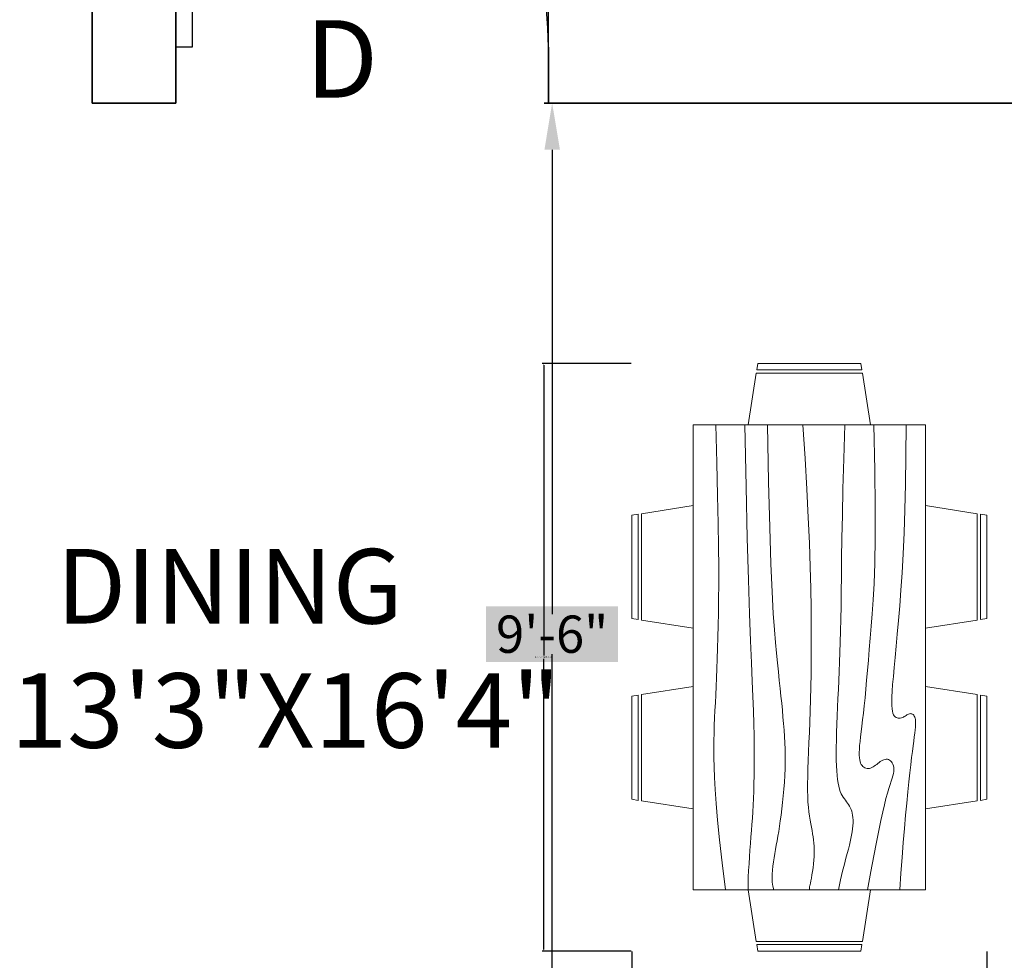
# Model space of a CAD drawing. Units: inches. Extents: x -128 to 854, y -395 to 398.
# Tile 36 of 61: x 164 to 270, y 95 to 196. Entities that reach past the tile are written whole.
import ezdxf

# ---------------------------------------------------------------- set-up
doc = ezdxf.new("R2010")
doc.units = ezdxf.units.IN
doc.header["$MEASUREMENT"] = 0
for name, color, linetype, lineweight in [('A-ANNO-DIMS', 2, 'Continuous', 18), ('A-ANNO-TEXT', 2, 'Continuous', 18), ('A-AREA-IDEN', 1, 'Continuous', 18), ('A-DOOR', 4, 'Continuous', 25), ('A-FURN', 8, 'Continuous', 18), ('A-WALL', 4, 'Continuous', 35)]:
    doc.layers.add(name, color=color, linetype=linetype, lineweight=lineweight)
doc.styles.get("Standard").update_dxf_attribs({"font": 'arial.ttf'})
doc.dimstyles.get("Standard").update_dxf_attribs({"dimtxt": 0.18, "dimasz": 0.18, "dimexe": 0.18, "dimexo": 0.0625, "dimgap": 0.09, "dimtad": 0, "dimtih": 1, "dimtoh": 1, "dimdec": 1, "dimzin": 0, "dimdsep": 46, "dimlunit": 4, "dimtxsty": 'Standard', "dimcen": 0.09, "dimclrd": 1, "dimclre": 2, "dimclrt": 6, "dimadec": 0, "dimazin": 0, "dimtfac": 1, "dimtdec": 1, "dimtofl": 0, "dimtmove": 0, "dimatfit": 3, "dimfxl": 1, "dimtfill": 2, "dimtfillclr": 3, "dimtolj": 1, "dimtzin": 0, "dimarcsym": 0})

# ---------------------------------------------------------------- blocks, each defined once
blk = doc.blocks.new('*U3')
for p, q in [((0, 0), (0, -6)), ((40, 0), (40, -6))]:
    blk.add_line(p, q)
blk.add_lwpolyline([(0, 0), (0, 40), (1.75, 40), (1.75, 0)], close=True)
blk.add_arc((0, 0), 40, 0, 90)
blk = doc.blocks.new('Dining Set - 36 x 72 in.')
for p, q in [((-22, 27.5), (-22.1562, 26.50042)), ((-22, 27.5), (-6, 27.5)), ((-5.8437, 26.49966), (-6, 27.5)), ((6, 27.5), (5.8438, 26.50042)), ((6, 27.5), (22, 27.5)), ((22.1563, 26.49966), (22, 27.5)), ((-22.2343, 26.00059), (-23.4847, 17.99762)), ((-22.2304, 26), (-5.7608, 26)), ((-5.8416, 26.5), (-22.1534, 26.5)), ((-4.5152, 17.99762), (-5.7655, 25.99926)), ((5.7657, 26.00059), (4.5153, 17.99762)), ((5.7696, 26), (22.2392, 26)), ((22.1584, 26.5), (5.8466, 26.5)), ((23.4848, 17.99762), (22.2345, 25.99926)), ((36, 18), (-36, 18)), ((-36, 18), (-36, -18)), ((36, -18), (36, 18)), ((-44.0006, 8.23428), (-35.9976, 9.48474)), ((44.0006, 8.23428), (35.9976, 9.48474)), ((-45.5, 8), (-44.5004, 8.15617)), ((-45.5, 8), (-45.5, -8)), ((-44.5, -8.15843), (-44.5, 8.15338)), ((-44, 8.23041), (-44, -8.23915)), ((44, 8.23041), (44, -8.23915)), ((44.5, -8.15843), (44.5, 8.15338)), ((45.5, 8), (44.5005, 8.15617)), ((45.5, 8), (45.5, -8)), ((-44.4997, -8.15631), (-45.5, -8)), ((-35.9976, -9.48476), (-43.9993, -8.2345)), ((35.9976, -9.48476), (43.9993, -8.2345)), ((44.4997, -8.15631), (45.5, -8)), ((-36, -18), (36, -18)), ((-22.2343, -26.0006), (-23.4847, -17.99762)), ((-4.5152, -17.99762), (-5.7655, -25.99928)), ((5.7657, -26.0006), (4.5153, -17.99762)), ((23.4848, -17.99762), (22.2345, -25.99928)), ((-22.2304, -26), (-5.7608, -26)), ((-22, -27.5), (-22.1562, -26.50044)), ((-5.8416, -26.5), (-22.1534, -26.5)), ((-5.8437, -26.49967), (-6, -27.5)), ((5.7696, -26), (22.2392, -26)), ((6, -27.5), (5.8438, -26.50044)), ((22.1584, -26.5), (5.8466, -26.5)), ((22.1563, -26.49967), (22, -27.5)), ((-22, -27.5), (-6, -27.5)), ((6, -27.5), (22, -27.5))]:
    blk.add_line(p, q)
for points in [[(-36, 15), (-31.1772, 14.97754), (-26.8079, 14.91406), (-22.8538, 14.81543), (-19.276, 14.6875), (-16.0362, 14.53613), (-13.0957, 14.36718), (-10.4159, 14.18652), (-7.9583, 14), (-5.6904, 13.81315), (-3.6035, 13.63021), (-1.6954, 13.45508), (0.0365, 13.29166), (1.5945, 13.14388), (2.9811, 13.01562), (4.1988, 12.9108), (5.25, 12.83333), (6.1393, 12.78613), (6.8802, 12.76823), (7.4883, 12.77767), (7.9792, 12.8125), (8.3685, 12.87077), (8.6719, 12.95052), (8.9049, 13.0498), (9.0833, 13.16666), (9.2205, 13.29899), (9.3216, 13.44401), (9.3895, 13.59879), (9.4271, 13.76041), (9.4373, 13.92594), (9.4232, 14.09245), (9.3875, 14.257), (9.3333, 14.41666), (9.2638, 14.56917), (9.1836, 14.71484), (9.0975, 14.85465), (9.0104, 14.98958), (8.9272, 15.1206), (8.8529, 15.2487), (8.7922, 15.37483), (8.75, 15.5), (8.7305, 15.62467), (8.7344, 15.74739), (8.7617, 15.86621), (8.8125, 15.97916), (8.8867, 16.08431), (8.9844, 16.17968), (9.1055, 16.26334), (9.25, 16.33333), (9.4189, 16.38802), (9.6172, 16.42708), (9.8506, 16.45052), (10.125, 16.45833), (10.4463, 16.45052), (10.8203, 16.42708), (11.2529, 16.38802), (11.75, 16.33333), (12.3184, 16.26318), (12.9694, 16.17838), (13.7151, 16.07991), (14.5677, 15.96875), (15.5395, 15.84586), (16.6426, 15.71224), (17.8893, 15.56884), (19.2917, 15.41666), (20.859, 15.25667), (22.5879, 15.08984), (24.4721, 14.91715), (26.5052, 14.73958), (28.6809, 14.5581), (30.9929, 14.3737), (33.4347, 14.18733), (36, 14)], [(-36, 10), (-28.9766, 10.14274), (-23.1725, 10.20442), (-18.4241, 10.19775), (-14.5677, 10.13541), (-11.4399, 10.03011), (-8.877, 9.89453), (-6.7154, 9.74137), (-4.7917, 9.58333), (-2.9698, 9.43082), (-1.2246, 9.28515), (0.4415, 9.14534), (2.026, 9.01041), (3.5266, 8.87939), (4.9408, 8.7513), (6.266, 8.62516), (7.5, 8.5), (8.6411, 8.37549), (9.6914, 8.2539), (10.6538, 8.13818), (11.5312, 8.03125), (12.3267, 7.93603), (13.043, 7.85547), (13.6831, 7.79248), (14.25, 7.75), (14.7471, 7.7303), (15.1797, 7.73307), (15.5537, 7.75732), (15.875, 7.80208), (16.1494, 7.86637), (16.3828, 7.94922), (16.5811, 8.04964), (16.75, 8.16666), (16.8944, 8.29915), (17.0143, 8.44531), (17.1089, 8.60319), (17.1771, 8.77083), (17.218, 8.94629), (17.2305, 9.1276), (17.2137, 9.31282), (17.1667, 9.5), (17.0895, 9.6875), (16.987, 9.875), (16.8649, 10.0625), (16.7292, 10.25), (16.5856, 10.4375), (16.4401, 10.625), (16.2985, 10.8125), (16.1667, 11), (16.05, 11.18733), (15.9518, 11.3737), (15.8752, 11.5581), (15.8229, 11.73958), (15.798, 11.91715), (15.8034, 12.08984), (15.842, 12.25667), (15.9167, 12.41666), (16.0295, 12.56836), (16.1784, 12.70833), (16.3605, 12.83268), (16.5729, 12.9375), (16.8127, 13.01888), (17.0768, 13.07291), (17.3625, 13.0957), (17.6667, 13.08333), (17.9894, 13.03312), (18.3418, 12.94726), (18.7382, 12.82918), (19.1927, 12.68229), (19.7195, 12.51001), (20.3327, 12.31575), (21.0465, 12.10294), (21.875, 11.875), (22.8357, 11.63354), (23.959, 11.37304), (25.2786, 11.08618), (26.8282, 10.76562), (28.6414, 10.40405), (30.752, 9.99414), (33.1936, 9.52856), (36, 9)], [(-36, 5.5), (-30.7157, 5.3348), (-26.069, 5.20963), (-21.9946, 5.11767), (-18.4271, 5.05208), (-15.3009, 5.00602), (-12.5508, 4.97265), (-10.1112, 4.94515), (-7.9167, 4.91666), (-5.909, 4.88167), (-4.0586, 4.83984), (-2.3429, 4.79215), (-0.7396, 4.73958), (0.7739, 4.6831), (2.22, 4.6237), (3.6213, 4.56233), (5, 4.5), (6.373, 4.43782), (7.7344, 4.3776), (9.0723, 4.32129), (10.375, 4.27083), (11.6309, 4.22819), (12.8281, 4.19531), (13.9551, 4.17415), (15, 4.16666), (15.954, 4.17448), (16.819, 4.19791), (17.6001, 4.23698), (18.3021, 4.29166), (18.9299, 4.36198), (19.4883, 4.44791), (19.9823, 4.54948), (20.4167, 4.66666), (20.7969, 4.79899), (21.1302, 4.94401), (21.4245, 5.09879), (21.6875, 5.26041), (21.9271, 5.42594), (22.1511, 5.59245), (22.3672, 5.757), (22.5834, 5.91666), (22.8065, 6.06868), (23.0404, 6.21093), (23.2879, 6.34147), (23.5521, 6.45833), (23.8358, 6.55957), (24.142, 6.64323), (24.4735, 6.70735), (24.8334, 6.75), (25.2235, 6.76969), (25.642, 6.76692), (26.0858, 6.74267), (26.5521, 6.69791), (27.0379, 6.63362), (27.5404, 6.55078), (28.0565, 6.45036), (28.5834, 6.33333), (29.1242, 6.19987), (29.7071, 6.04687), (30.3661, 5.87044), (31.1354, 5.66666), (32.0493, 5.43164), (33.142, 5.16146), (34.4475, 4.85221), (36, 4.5)], [(-36, -1), (-30.7915, -0.6591), (-26.0195, -0.38216), (-21.6519, -0.16284), (-17.6563, 0.00521), (-14.0005, 0.12833), (-10.6523, 0.21289), (-7.5796, 0.26522), (-4.75, 0.29166), (-2.134, 0.29793), (0.2878, 0.28711), (2.5317, 0.26163), (4.6146, 0.22396), (6.5529, 0.17651), (8.3633, 0.12174), (10.0623, 0.06209), (11.6667, 0), (13.1899, -0.06201), (14.6341, -0.1211), (15.9982, -0.17432), (17.2813, -0.21875), (18.4823, -0.25147), (19.6003, -0.26953), (20.6343, -0.27002), (21.5834, -0.25), (22.4481, -0.20768), (23.2357, -0.14584), (23.9549, -0.06836), (24.6146, 0.02083), (25.2235, 0.11784), (25.7904, 0.21875), (26.3241, 0.31966), (26.8334, 0.41666), (27.3265, 0.50618), (27.8099, 0.58593), (28.2894, 0.65397), (28.7709, 0.70833), (29.2601, 0.74707), (29.763, 0.76823), (30.2855, 0.76985), (30.8334, 0.75), (31.4088, 0.70784), (31.9994, 0.64713), (32.589, 0.57275), (33.1615, 0.48958), (33.7008, 0.4025), (34.1908, 0.3164), (34.6153, 0.23616), (34.9584, 0.16666), (35.2099, 0.11165), (35.3848, 0.07031), (35.504, 0.04069), (35.5886, 0.02083), (35.6594, 0.00879), (35.7377, 0.0026), (35.8442, 0.00032), (36, 0)], [(-36, -6.5), (-27.1843, -6.31267), (-20.084, -6.1263), (-14.469, -5.9419), (-10.1094, -5.76042), (-6.7752, -5.58285), (-4.2363, -5.41016), (-2.2629, -5.24333), (-0.625, -5.08334), (0.8708, -4.93099), (2.2715, -4.78646), (3.5872, -4.64974), (4.8281, -4.52084), (6.0046, -4.39974), (7.127, -4.28646), (8.2053, -4.18099), (9.25, -4.08334), (10.2705, -3.99382), (11.2734, -3.91407), (12.2647, -3.84603), (13.25, -3.79167), (14.2354, -3.75293), (15.2266, -3.73177), (16.2295, -3.73015), (17.25, -3.75), (18.2912, -3.79248), (19.3451, -3.85547), (20.4009, -3.93604), (21.4479, -4.03125), (22.4754, -4.13819), (23.4727, -4.25391), (24.4289, -4.37549), (25.3334, -4.5), (26.1785, -4.62492), (26.9694, -4.74935), (27.7145, -4.87281), (28.4219, -4.99479), (29.1, -5.11483), (29.7572, -5.23242), (30.4016, -5.34709), (31.0417, -5.45834), (31.6837, -5.56437), (32.3262, -5.65821), (32.9658, -5.73153), (33.599, -5.77604), (34.2224, -5.78345), (34.8327, -5.74545), (35.4264, -5.65373), (36, -5.5)], [(-36, -10), (-26.4022, -9.81299), (-18.4675, -9.62891), (-11.9839, -9.45069), (-6.7396, -9.28125), (-2.5226, -9.12354), (0.8789, -8.98047), (3.6769, -8.85498), (6.0833, -8.75), (8.2767, -8.66765), (10.3021, -8.60677), (12.1712, -8.56543), (13.8958, -8.54167), (15.4876, -8.53353), (16.9583, -8.53907), (18.3197, -8.55632), (19.5834, -8.58334), (20.7616, -8.61841), (21.8685, -8.66081), (22.9188, -8.71004), (23.9271, -8.76563), (24.9081, -8.82707), (25.8763, -8.89388), (26.8465, -8.96558), (27.8334, -9.04167), (28.8474, -9.12118), (29.8828, -9.20117), (30.93, -9.27824), (31.9792, -9.34896), (33.0205, -9.40991), (34.0443, -9.45768), (35.0407, -9.48885), (36, -9.5)], [(-36, -14.5), (-30.0881, -14.33513), (-25.0332, -14.21224), (-20.7312, -14.12647), (-17.0781, -14.07292), (-13.97, -14.04671), (-11.3027, -14.04297), (-8.9724, -14.05681), (-6.875, -14.08334), (-4.9224, -14.11833), (-3.0905, -14.16016), (-1.3709, -14.20785), (0.2448, -14.26042), (1.7647, -14.3169), (3.1973, -14.3763), (4.5507, -14.43767), (5.8333, -14.5), (7.0554, -14.5621), (8.235, -14.62175), (9.3922, -14.67652), (10.5469, -14.72396), (11.7192, -14.76164), (12.929, -14.78711), (14.1965, -14.79794), (15.5417, -14.79167), (16.9933, -14.76424), (18.6152, -14.70508), (20.4804, -14.60197), (22.6615, -14.44271), (25.2312, -14.21509), (28.2624, -13.9069), (31.8277, -13.50594), (36, -13)]]:
    blk.add_lwpolyline(points)
blk = doc.blocks.new('*D55')
at = {"layer": 'A-ANNO-DIMS', "color": 0, "lineweight": -2, "transparency": 16777216}
for p, q in [((304.81, 186.74), (221.09, 186.74)), ((221.27, 181.74), (221.27, 131.87)), ((221.27, 77.74), (221.27, 127.61)), ((304.81, 72.74), (221.09, 72.74))]:
    blk.add_line(p, q, dxfattribs=at)
at = {"layer": 'A-ANNO-DIMS', "color": 0, "transparency": 16777216}
for points in [[(220.44, 181.74), (222.11, 181.74), (221.27, 186.74)], [(220.44, 77.74), (222.11, 77.74), (221.27, 72.74)]]:
    blk.add_solid(points, dxfattribs=at)
at = {"layer": 'Defpoints', "color": 0, "transparency": 16777216}
for p in [(221.27, 186.74), (304.87, 186.74), (304.87, 72.74)]:
    blk.add_point(p, dxfattribs=at)
at = {"layer": 'A-ANNO-DIMS', "color": 0, "transparency": 16777216, "insert": (221.27, 129.74), "char_height": 4, "attachment_point": 5, "bg_fill": 1, "box_fill_scale": 1.25, "bg_fill_color": 3, "bg_fill_transparency": 0}
blk.add_mtext('\\A1;9\'-6"', dxfattribs=at)
blk = doc.blocks.new('*D91')
at = {"layer": 'A-ANNO-DIMS', "color": 2, "lineweight": -2, "transparency": 16777216}
for p, q in [((229.77, 158.8), (220.19, 158.8)), ((229.77, 95.73), (220.19, 95.73))]:
    blk.add_line(p, q, dxfattribs=at)
at = {"layer": 'A-ANNO-DIMS', "color": 1, "lineweight": -2, "transparency": 16777216}
for p, q in [((220.37, 158.62), (220.37, 127.45)), ((220.37, 95.91), (220.37, 127.08))]:
    blk.add_line(p, q, dxfattribs=at)
at = {"layer": 'A-ANNO-DIMS', "color": 1, "transparency": 16777216}
for points in [[(220.34, 158.62), (220.4, 158.62), (220.37, 158.8)], [(220.34, 95.91), (220.4, 95.91), (220.37, 95.73)]]:
    blk.add_solid(points, dxfattribs=at)
at = {"layer": 'Defpoints', "color": 0, "transparency": 16777216}
for p in [(229.83, 158.8), (220.37, 95.73), (229.83, 95.73)]:
    blk.add_point(p, dxfattribs=at)
at = {"layer": 'A-ANNO-DIMS', "color": 6, "transparency": 16777216, "insert": (220.37, 127.26), "char_height": 0.18, "attachment_point": 5, "bg_fill": 1, "box_fill_scale": 1.25, "bg_fill_color": 3, "bg_fill_transparency": 0}
blk.add_mtext('\\A1;DINING SET 5\'-3"', dxfattribs=at)
blk = doc.blocks.new('*D92')
at = {"layer": 'A-ANNO-DIMS', "color": 2, "lineweight": -2, "transparency": 16777216}
for p, q in [((229.83, 95.67), (229.83, 86.09)), ((267.95, 95.67), (267.95, 86.09))]:
    blk.add_line(p, q, dxfattribs=at)
at = {"layer": 'A-ANNO-DIMS', "color": 1, "lineweight": -2, "transparency": 16777216}
for p, q in [((230.01, 86.27), (248.56, 86.27)), ((267.77, 86.27), (249.22, 86.27))]:
    blk.add_line(p, q, dxfattribs=at)
at = {"layer": 'A-ANNO-DIMS', "color": 1, "transparency": 16777216}
for points in [[(230.01, 86.3), (230.01, 86.24), (229.83, 86.27)], [(267.77, 86.3), (267.77, 86.24), (267.95, 86.27)]]:
    blk.add_solid(points, dxfattribs=at)
at = {"layer": 'Defpoints', "color": 0, "transparency": 16777216}
for p in [(229.83, 95.73), (267.95, 95.73), (267.95, 86.27)]:
    blk.add_point(p, dxfattribs=at)
at = {"layer": 'A-ANNO-DIMS', "color": 6, "transparency": 16777216, "insert": (248.89, 86.27), "char_height": 0.18, "attachment_point": 5, "bg_fill": 1, "box_fill_scale": 1.25, "bg_fill_color": 3, "bg_fill_transparency": 0}
blk.add_mtext('\\A1;3\'-2"', dxfattribs=at)
blk = doc.blocks.new('*D101')
at = {"layer": 'A-ANNO-DIMS', "color": 2, "lineweight": -2, "transparency": 16777216}
for p, q in [((180.87, 186.8), (180.87, 386.74)), ((220.87, 186.8), (220.87, 386.74))]:
    blk.add_line(p, q, dxfattribs=at)
at = {"layer": 'A-ANNO-DIMS', "color": 1, "lineweight": -2, "transparency": 16777216}
for p, q in [((181.05, 386.56), (200.54, 386.56)), ((220.69, 386.56), (201.2, 386.56))]:
    blk.add_line(p, q, dxfattribs=at)
at = {"layer": 'A-ANNO-DIMS', "color": 1, "transparency": 16777216}
for points in [[(181.05, 386.59), (181.05, 386.53), (180.87, 386.56)], [(220.69, 386.59), (220.69, 386.53), (220.87, 386.56)]]:
    blk.add_solid(points, dxfattribs=at)
at = {"layer": 'Defpoints', "color": 0, "transparency": 16777216}
for p in [(220.87, 386.56), (180.87, 186.74), (220.87, 186.74)]:
    blk.add_point(p, dxfattribs=at)
at = {"layer": 'A-ANNO-DIMS', "color": 6, "transparency": 16777216, "insert": (200.87, 386.56), "char_height": 0.18, "attachment_point": 5, "bg_fill": 1, "box_fill_scale": 1.25, "bg_fill_color": 3, "bg_fill_transparency": 0}
blk.add_mtext('\\A1;3\'-4"', dxfattribs=at)

msp = doc.modelspace()

# ---------------------------------------------------------------- linework, layer by layer
at = {"layer": 'A-WALL'}
for p, q in [((180.87, 339.74), (180.87, 186.74)), ((171.87, 210.74), (171.87, 186.74)), ((180.87, 186.74), (171.87, 186.74)), ((304.87, 186.74), (220.42, 186.74))]:
    msp.add_line(p, q, dxfattribs=at)

# ---------------------------------------------------------------- block references
at = {"layer": 'A-DOOR'}
msp.add_blockref('*U3', (180.87, 192.74), dxfattribs=at)
at = {"layer": 'A-FURN', "xscale": 0.6930679910976857, "yscale": 0.6930679910976857, "zscale": 0.6930679910976857, "rotation": 270}
msp.add_blockref('Dining Set - 36 x 72 in.', (248.89, 127.26), dxfattribs=at)

# ---------------------------------------------------------------- texts
at = {"layer": 'A-ANNO-TEXT'}
msp.add_text('D', height=8.31, dxfattribs=at).set_placement((194.78, 187.33))
at = {"layer": 'A-AREA-IDEN', "insert": (163.13, 138.88), "char_height": 8, "attachment_point": 1}
msp.add_mtext_dynamic_manual_height_columns('  DINING\\P13\'3"X16\'4"', width=99.0352, gutter_width=1, heights=[0], dxfattribs=at)

# ---------------------------------------------------------------- dimensions: what is measured, and where the dimension line sits
at = {"layer": 'A-ANNO-DIMS'}
for base, p1, p2, picture, middle in [((220.87, 386.56), (180.87, 186.74), (220.87, 186.74), '*D101', (200.87, 386.56)), ((267.95, 86.27), (229.83, 95.73), (267.95, 95.73), '*D92', (248.89, 86.27))]:
    dim = msp.add_linear_dim(base=base, p1=p1, p2=p2, dimstyle='Standard', override={"dimdec": 1, "dimlfac": 1, "dimrnd": 0, "dimzin": 1, "dimdsep": 46, "dimlunit": 4, "dimfrac": 2}, dxfattribs=at)
    dim.commit()
    dim.dimension.update_dxf_attribs({"geometry": picture, "text_midpoint": middle})
dim = msp.add_linear_dim(base=(221.27, 186.74), p1=(304.87, 72.74), p2=(304.87, 186.74), angle=90, dimstyle='Standard', override={"dimtxt": 4, "dimasz": 5, "dimclrd": 0, "dimclre": 0, "dimclrt": 0}, dxfattribs=at)
dim.commit()
dim.dimension.update_dxf_attribs({"geometry": '*D55', "text_midpoint": (221.27, 129.74)})
dim = msp.add_linear_dim(base=(220.37, 95.73), p1=(229.83, 158.8), p2=(229.83, 95.73), angle=270, text='DINING SET <>', dimstyle='Standard', override={"dimdec": 1, "dimlfac": 1, "dimrnd": 0, "dimzin": 1, "dimdsep": 46, "dimlunit": 4, "dimfrac": 2}, dxfattribs=at)
dim.commit()
dim.dimension.update_dxf_attribs({"geometry": '*D91', "text_midpoint": (220.37, 127.26)})

doc.saveas('drawing.dxf')
